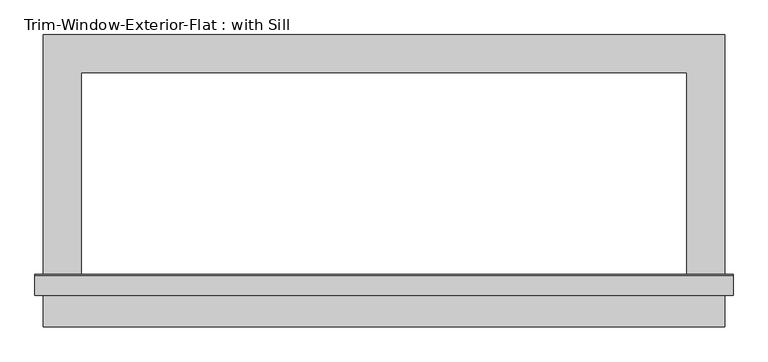
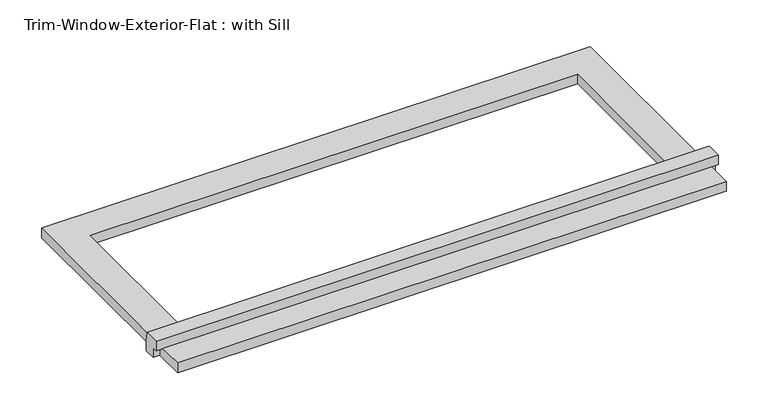
"""IFC4 building model written with IfcOpenShell, lengths in millimetres: proxy geometry, Trim-Window-Exterior-Flat : with Sill."""

from ifc_helpers import new_model, si_unit, frame, origin, origin_with_axes, place, context, project, spatial, polyline, outline, extrude, source, transform, mapped, element, save


def trim_window_exterior_flat_with_sill_3de9c0e0(model_context):
    return source(origin(), model_context, "Body", "SweptSolid", [
        extrude(outline(polyline([(514.35, -326.9823709), (514.35, -384.1323709), (-514.35, -384.1323709), (-514.35, -326.9823709), (514.35, -326.9823709)])), origin_with_axes(), (0.0, 0.0, 1.0), 19.05),
        extrude(outline(polyline([(-336.55, 38.1), (-307.2580645, 38.1), (-304.8, 19.05), (-304.8, 0.0), (-326.9823709, 0.0), (-326.9823709, 19.05), (-336.55, 19.05), (-336.55, 38.1)])), frame((-527.05, 0.0, 0.0), z_axis=(1.0, 0.0, 0.0), x_axis=(0.0, 1.0, 0.0)), (0.0, 0.0, 1.0), 1054.1),
        extrude(outline(polyline([(-514.35, 57.15), (514.35, 57.15), (514.35, -304.8), (457.2, -304.8), (457.2, 0.0), (-457.2, 0.0), (-457.2, -304.8), (-514.35, -304.8), (-514.35, 57.15)])), origin_with_axes(), (0.0, 0.0, 1.0), 19.05),
    ])


if __name__ == "__main__":
    model = new_model("IFC4")
    model_context = context("Model", 3, world=origin())
    ifc_project = project(units=[si_unit("LENGTHUNIT", "METRE", prefix="MILLI")], contexts=[model_context])
    site = spatial("IfcSite", under=ifc_project)
    building = spatial("IfcBuilding", under=site)
    placement = place(None, origin())
    trim_window_exterior_flat_with_sill_shape = trim_window_exterior_flat_with_sill_3de9c0e0(model_context)
    element("IfcBuildingElementProxy", 1, Name="Trim-Window-Exterior-Flat : with Sill", ObjectType="Trim-Window-Exterior-Flat : with Sill", at=placement, inside=building, context=model_context, shape_type="MappedRepresentation", body=[
        mapped(trim_window_exterior_flat_with_sill_shape, transform((0.0, 0.0, 0.0), x_axis=(1.0, 0.0, 0.0), y_axis=(0.0, 1.0, 0.0), z_axis=(0.0, 0.0, 1.0))),
    ])
    save(model, "model.ifc")

# Revit data of these elements
# Type "Trim-Window-Exterior-Flat : with Sill"
#   Trim Width = 0' - 2 1/4"
#   Trim Thickness_Picture Frame = 0' - 1 1/4"
#   Trim Thickness_with Sill = 0' - 0 3/4"
#   Sill Thickness = 0' - 1 1/4"
#   Opening Width [instance default] = 2' - 0"
#   Opening Height [instance default] = 3' - 0"
#   Default Elevation = 4' - 0"
#   Sill = yes
#   Picture Frame = no
#   Trim Material [instance default] = none
# Element 1 (IfcBuildingElementProxy, "Trim-Window-Exterior-Flat : with Sill")
#   Opening Width = 3' - 0"
#   Opening Height = 1' - 0"
#   Trim Material = Clad - White
#   Materials on its faces: "Clad - White"
# Materials
#   "Clad - White": class "Wood", colour RGB 242 242 238, transparency 0, Cost = 0
